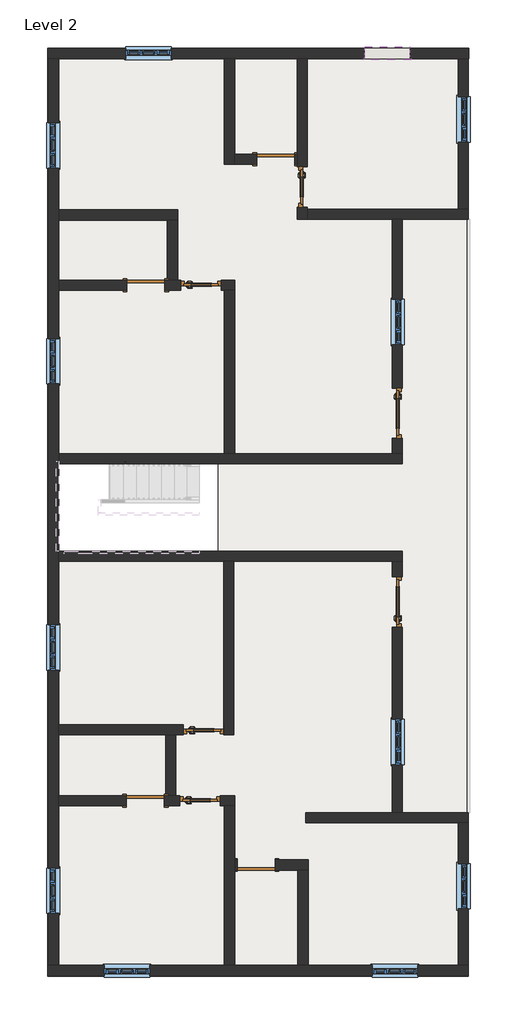
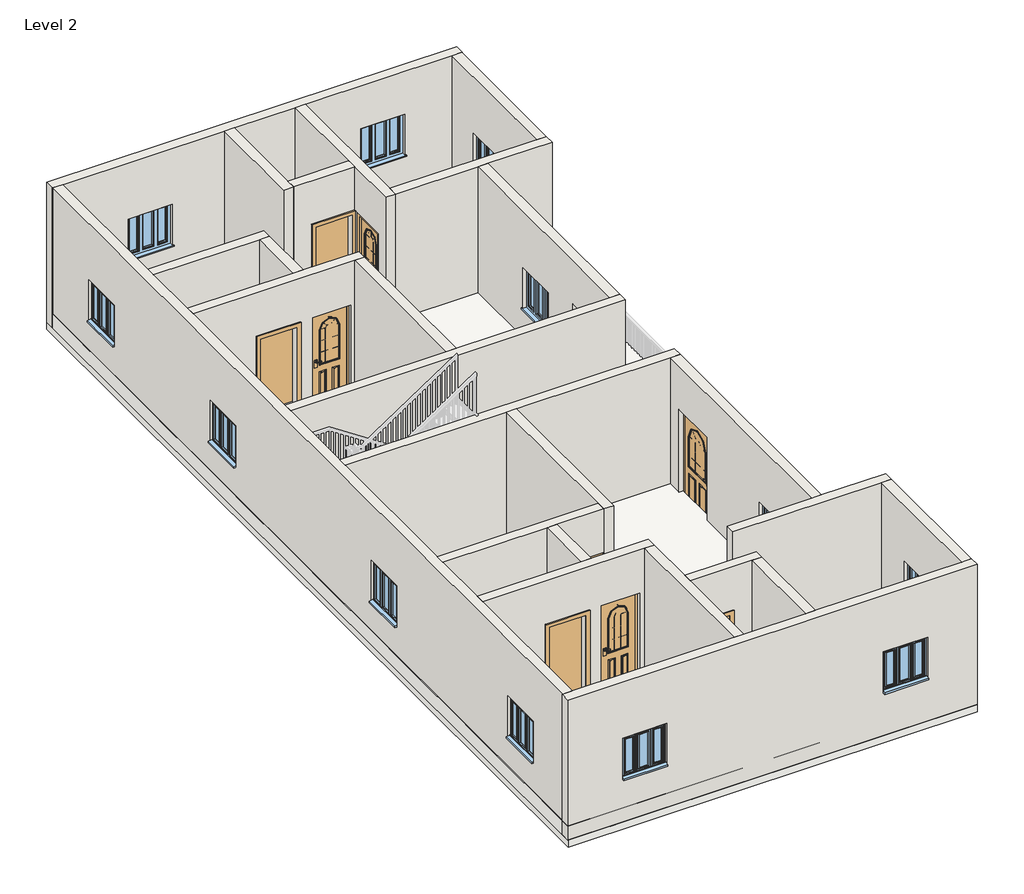
# One storey, part 1 of 3: 25 walls, 12 windows, 10 doors, 1 roof, 1 slab.
"""IFC4 building model written with IfcOpenShell, lengths in millimetres."""

from ifc_helpers import new_model, si_unit, frame, origin, place, context, project, spatial, polyline, outline, extrude, faceted_brep, transform, mapped, element, save
from components import doors_extsgl_w_glazing_bars_arched_1010x2110mm_bccdb1b2, doors_extsgl_w_glazing_bars_arched_1010x2110mm_5c897e1f, doors_extsgl_w_glazing_bars_arched_810x2110mm_57ea6d9e, doors_extsgl_w_glazing_bars_arched_810x2110mm_84a0a083, door_fadea3f2, windows_tpl_w_glazing_bars_910x910mm_9d987a72

model = new_model("IFC4")

# Units and contexts
model_context = context("Model", 3, world=origin())
ifc_project = project(units=[si_unit("LENGTHUNIT", "METRE", prefix="MILLI")], contexts=[model_context])

# Site, building, storey
site = spatial("IfcSite", under=ifc_project)
building = spatial("IfcBuilding", under=site)
storey = spatial("IfcBuildingStorey", under=building, Name="Level 2", Elevation=3048.0)

# Doors
placement = place(None, origin())
doors_extsgl_w_glazing_bars_arched_1010x2110mm_shape = doors_extsgl_w_glazing_bars_arched_1010x2110mm_bccdb1b2(model_context)
element("IfcDoor", 1, ObjectType="Doors_ExtSgl_w-Glazing_Bars_Arched : 1010x2110mm", at=placement, inside=storey, context=model_context, shape_type="MappedRepresentation", body=[
    mapped(doors_extsgl_w_glazing_bars_arched_1010x2110mm_shape, transform((1850.5605895, 2208.5797121, 3048.0), x_axis=(0.0, -1.0, 0.0), y_axis=(1.0, 0.0, 0.0), z_axis=(0.0, 0.0, 1.0))),
])
doors_extsgl_w_glazing_bars_arched_1010x2110mm_2_shape = doors_extsgl_w_glazing_bars_arched_1010x2110mm_5c897e1f(model_context)
element("IfcDoor", 2, ObjectType="Doors_ExtSgl_w-Glazing_Bars_Arched : 1010x2110mm", at=placement, inside=storey, context=model_context, shape_type="MappedRepresentation", body=[
    mapped(doors_extsgl_w_glazing_bars_arched_1010x2110mm_2_shape, transform((1850.5605895, -1576.0202879, 3048.0), x_axis=(0.0, 1.0, 0.0), y_axis=(-1.0, 0.0, 0.0), z_axis=(0.0, 0.0, 1.0))),
])
doors_extsgl_w_glazing_bars_arched_810x2110mm_shape = doors_extsgl_w_glazing_bars_arched_810x2110mm_57ea6d9e(model_context)
element("IfcDoor", 3, ObjectType="Doors_ExtSgl_w-Glazing_Bars_Arched : 810x2110mm", at=placement, inside=storey, context=model_context, shape_type="MappedRepresentation", body=[
    mapped(doors_extsgl_w_glazing_bars_arched_810x2110mm_shape, transform((-2086.4394105, 4773.9797121, 3048.0), x_axis=(1.0, 0.0, 0.0), y_axis=(0.0, 1.0, 0.0), z_axis=(0.0, 0.0, 1.0))),
])
element("IfcDoor", 4, ObjectType="Doors_ExtSgl_w-Glazing_Bars_Arched : 810x2110mm", at=placement, inside=storey, context=model_context, shape_type="MappedRepresentation", body=[
    mapped(doors_extsgl_w_glazing_bars_arched_810x2110mm_shape, transform((-2105.4894105, -5563.8202879, 3048.0), x_axis=(1.0, 0.0, 0.0), y_axis=(0.0, 1.0, 0.0), z_axis=(0.0, 0.0, 1.0))),
])
doors_extsgl_w_glazing_bars_arched_810x2110mm_2_shape = doors_extsgl_w_glazing_bars_arched_810x2110mm_84a0a083(model_context)
element("IfcDoor", 5, ObjectType="Doors_ExtSgl_w-Glazing_Bars_Arched : 810x2110mm", at=placement, inside=storey, context=model_context, shape_type="MappedRepresentation", body=[
    mapped(doors_extsgl_w_glazing_bars_arched_810x2110mm_2_shape, transform((-2035.6394105, -4141.4202879, 3048.0), x_axis=(1.0, 0.0, 0.0), y_axis=(0.0, 1.0, 0.0), z_axis=(0.0, 0.0, 1.0))),
])
element("IfcDoor", 6, ObjectType="Doors_ExtSgl_w-Glazing_Bars_Arched : 810x2110mm", at=placement, inside=storey, context=model_context, shape_type="MappedRepresentation", body=[
    mapped(doors_extsgl_w_glazing_bars_arched_810x2110mm_2_shape, transform((-54.4394105, 6748.5640518, 3048.0), x_axis=(0.0, -1.0, 0.0), y_axis=(1.0, 0.0, 0.0), z_axis=(0.0, 0.0, 1.0))),
])
door_shape = door_fadea3f2(model_context)
element("IfcDoor", 7, ObjectType="Single-Flush : 30\" x 80\"", at=placement, inside=storey, context=model_context, shape_type="MappedRepresentation", body=[
    mapped(door_shape, transform((-3204.0394105, -5563.8202879, 3048.0), x_axis=(1.0, 0.0, 0.0), y_axis=(0.0, 1.0, 0.0), z_axis=(0.0, 0.0, 1.0))),
])
element("IfcDoor", 8, ObjectType="Single-Flush : 30\" x 80\"", at=placement, inside=storey, context=model_context, shape_type="MappedRepresentation", body=[
    mapped(door_shape, transform((-981.5394105, -6850.9128362, 3048.0), x_axis=(-1.0, 0.0, 0.0), y_axis=(0.0, -1.0, 0.0), z_axis=(0.0, 0.0, 1.0))),
])
element("IfcDoor", 9, ObjectType="Single-Flush : 30\" x 80\"", at=placement, inside=storey, context=model_context, shape_type="MappedRepresentation", body=[
    mapped(door_shape, transform((-3191.3394105, 4773.9797121, 3048.0), x_axis=(1.0, 0.0, 0.0), y_axis=(0.0, 1.0, 0.0), z_axis=(0.0, 0.0, 1.0))),
])
element("IfcDoor", 10, ObjectType="Single-Flush : 30\" x 80\"", at=placement, inside=storey, context=model_context, shape_type="MappedRepresentation", body=[
    mapped(door_shape, transform((-587.8394105, 7301.2797121, 3048.0), x_axis=(1.0, 0.0, 0.0), y_axis=(0.0, 1.0, 0.0), z_axis=(0.0, 0.0, 1.0))),
])

# Roof
element("IfcRoof", 11, ObjectType="Generic - 12\"", at=placement, inside=storey, context=model_context, shape_type="SweptSolid", body=[
    extrude(outline(polyline([(3272.9605895, 9523.7797121), (3272.9605895, -9069.0202879), (-5159.8394105, -9069.0202879), (-5159.8394105, 9523.7797121), (3272.9605895, 9523.7797121)]), holes=[polyline([(-1756.1922756, 1192.5797121), (-4943.9394105, 1192.5797121), (-4943.9394105, -560.0202879), (-1756.1922756, -560.0202879), (-1756.1922756, 1192.5797121)])]), frame((0.0, 0.0, 3048.0), z_axis=(0.0, 0.0, 1.0), x_axis=(1.0, 0.0, 0.0)), (0.0, 0.0, 1.0), 304.8),
])

# Slab
element("IfcSlab", 12, ObjectType="Generic - 12\"", at=placement, inside=storey, context=model_context, shape_type="SweptSolid", body=[
    extrude(outline(polyline([(3272.9605895, 9523.7797121), (3272.9605895, -9081.7202879), (-5159.8394105, -9081.7202879), (-5159.8394105, 9523.7797121), (3272.9605895, 9523.7797121)]), holes=[polyline([(-1756.1922756, 1192.5797121), (-4943.9394105, 1192.5797121), (-4943.9394105, -560.0202879), (-1756.1922756, -560.0202879), (-1756.1922756, 1192.5797121)])]), frame((0.0, 0.0, 2895.6), z_axis=(0.0, 0.0, 1.0), x_axis=(1.0, 0.0, 0.0)), (0.0, 0.0, 1.0), 152.4),
])

# Walls
element("IfcWall", 13, ObjectType="Generic - 4.5\" p", at=placement, inside=storey, context=model_context, shape_type="Brep", body=[
    faceted_brep([(-2810.3394105, 4672.3797121, 5080.0), (-2810.3394105, 4672.3797121, 3048.0), (-2491.4394105, 4672.3797121, 3048.0), (-2491.4394105, 4672.3797121, 5158.0), (-1681.4394105, 4672.3797121, 5158.0), (-1681.4394105, 4672.3797121, 3048.0), (-1616.5394105, 4672.3797121, 3048.0), (-1413.3394105, 4672.3797121, 3048.0), (-1413.3394105, 4672.3797121, 6096.0), (-1616.5394105, 4672.3797121, 6096.0), (-4943.9394105, 4672.3797121, 6096.0), (-4943.9394105, 4672.3797121, 3048.0), (-3572.3394105, 4672.3797121, 3048.0), (-3572.3394105, 4672.3797121, 5080.0), (-2491.4394105, 4875.5797121, 3048.0), (-2556.3394105, 4875.5797121, 3048.0), (-2759.5394105, 4875.5797121, 3048.0), (-2810.3394105, 4875.5797121, 3048.0), (-2810.3394105, 4875.5797121, 5080.0), (-3572.3394105, 4875.5797121, 5080.0), (-3572.3394105, 4875.5797121, 3048.0), (-4943.9394105, 4875.5797121, 3048.0), (-4943.9394105, 4875.5797121, 6096.0), (-2759.5394105, 4875.5797121, 6096.0), (-2556.3394105, 4875.5797121, 6096.0), (-1413.3394105, 4875.5797121, 6096.0), (-1413.3394105, 4875.5797121, 3048.0), (-1681.4394105, 4875.5797121, 3048.0), (-1681.4394105, 4875.5797121, 5158.0), (-2491.4394105, 4875.5797121, 5158.0)], [[[0, 1, 2, 3, 4, 5, 6, 7, 8, 9, 10, 11, 12, 13]], [[14, 15, 16, 17, 18, 19, 20, 21, 22, 23, 24, 25, 26, 27, 28, 29]], [[7, 6, 5, 27, 26]], [[12, 11, 21, 20]], [[2, 1, 17, 16, 15, 14]], [[10, 9, 8, 25, 24, 23, 22]], [[11, 10, 22, 21]], [[8, 7, 26, 25]], [[14, 29, 3, 2]], [[28, 27, 5, 4]], [[29, 28, 4, 3]], [[18, 17, 1, 0]], [[19, 18, 0, 13]], [[20, 19, 13, 12]]]),
])
element("IfcWall", 14, ObjectType="Generic - 4.5\" p", at=placement, inside=storey, context=model_context, shape_type="SweptSolid", body=[
    extrude(outline(polyline([(-1616.5394105, 1395.7797121), (-1616.5394105, 4672.3797121), (-1413.3394105, 4672.3797121), (-1413.3394105, 1395.7797121), (-1616.5394105, 1395.7797121)])), frame((0.0, 0.0, 3048.0), z_axis=(0.0, 0.0, 1.0), x_axis=(1.0, 0.0, 0.0)), (0.0, 0.0, 1.0), 3048.0),
])
element("IfcWall", 15, ObjectType="Generic - 4.5\" p", at=placement, inside=storey, context=model_context, shape_type="Brep", body=[
    faceted_brep([(-4943.9394105, 6082.1542467, 3048.0), (-2759.5394105, 6082.1542467, 3048.0), (-2556.3394105, 6082.1542467, 3048.0), (-2556.3394105, 6082.1542467, 6096.0), (-2759.5394105, 6082.1542467, 6096.0), (-4943.9394105, 6082.1542467, 6096.0), (-4943.9394105, 6285.3542467, 3048.0), (-4943.9394105, 6285.3542467, 6096.0), (-2556.3394105, 6285.3542467, 6096.0), (-2556.3394105, 6285.3542467, 3048.0)], [[[0, 1, 2, 3, 4, 5]], [[6, 7, 8, 9]], [[2, 1, 0, 6, 9]], [[5, 4, 3, 8, 7]], [[0, 5, 7, 6]], [[3, 2, 9, 8]]]),
])
element("IfcWall", 16, ObjectType="Generic - 4.5\" p", at=placement, inside=storey, context=model_context, shape_type="SweptSolid", body=[
    extrude(outline(polyline([(-2759.5394105, 4875.5797121), (-2759.5394105, 6082.1542467), (-2556.3394105, 6082.1542467), (-2556.3394105, 4875.5797121), (-2759.5394105, 4875.5797121)])), frame((0.0, 0.0, 3048.0), z_axis=(0.0, 0.0, 1.0), x_axis=(1.0, 0.0, 0.0)), (0.0, 0.0, 1.0), 3048.0),
])
element("IfcWall", 17, ObjectType="Generic - 4.5\" p", at=placement, inside=storey, context=model_context, shape_type="Brep", body=[
    faceted_brep([(-1616.5394105, 9320.5797121, 3048.0), (-1616.5394105, 7199.6797121, 3048.0), (-1616.5394105, 7199.6797121, 6096.0), (-1616.5394105, 9320.5797121, 6096.0), (-1413.3394105, 9320.5797121, 3048.0), (-1413.3394105, 9320.5797121, 6096.0), (-1413.3394105, 7402.8797121, 6096.0), (-1413.3394105, 7199.6797121, 6096.0), (-1413.3394105, 7199.6797121, 3048.0), (-1413.3394105, 7402.8797121, 3048.0)], [[[0, 1, 2, 3]], [[4, 5, 6, 7, 8, 9]], [[1, 0, 4, 9, 8]], [[3, 2, 7, 6, 5]], [[0, 3, 5, 4]], [[2, 1, 8, 7]]]),
])
element("IfcWall", 18, ObjectType="Generic - 4.5\" p", at=placement, inside=storey, context=model_context, shape_type="SweptSolid", body=[
    extrude(outline(polyline([(5080.0, -206.8394105), (3048.0, -206.8394105), (3048.0, -156.0394105), (6096.0, -156.0394105), (6096.0, -1413.3394105), (3048.0, -1413.3394105), (3048.0, -968.8394105), (5080.0, -968.8394105), (5080.0, -206.8394105)])), frame((0.0, 7199.6797121, 0.0), z_axis=(0.0, 1.0, 0.0), x_axis=(0.0, 0.0, 1.0)), (0.0, 0.0, 1.0), 203.2),
])
element("IfcWall", 19, ObjectType="Generic - 4.5\" p", at=placement, inside=storey, context=model_context, shape_type="Brep", body=[
    faceted_brep([(-156.0394105, 6343.5640518, 5158.0), (-156.0394105, 6343.5640518, 3048.0), (-156.0394105, 6094.2483916, 3048.0), (-156.0394105, 6094.2483916, 6096.0), (-156.0394105, 7199.6797121, 6096.0), (-156.0394105, 7402.8797121, 6096.0), (-156.0394105, 9320.5797121, 6096.0), (-156.0394105, 9320.5797121, 3048.0), (-156.0394105, 7402.8797121, 3048.0), (-156.0394105, 7199.6797121, 3048.0), (-156.0394105, 7153.5640518, 3048.0), (-156.0394105, 7153.5640518, 5158.0), (47.1605895, 6094.2483916, 3048.0), (47.1605895, 6297.4483916, 3048.0), (47.1605895, 6343.5640518, 3048.0), (47.1605895, 6343.5640518, 5158.0), (47.1605895, 7153.5640518, 5158.0), (47.1605895, 7153.5640518, 3048.0), (47.1605895, 9320.5797121, 3048.0), (47.1605895, 9320.5797121, 6096.0), (47.1605895, 6297.4483916, 6096.0), (47.1605895, 6094.2483916, 6096.0)], [[[0, 1, 2, 3, 4, 5, 6, 7, 8, 9, 10, 11]], [[12, 13, 14, 15, 16, 17, 18, 19, 20, 21]], [[2, 1, 14, 13, 12]], [[10, 9, 8, 7, 18, 17]], [[6, 5, 4, 3, 21, 20, 19]], [[7, 6, 19, 18]], [[3, 2, 12, 21]], [[17, 16, 11, 10]], [[15, 14, 1, 0]], [[16, 15, 0, 11]]]),
])
element("IfcWall", 20, ObjectType="Generic - 4.5\" p", at=placement, inside=storey, context=model_context, shape_type="Brep", body=[
    faceted_brep([(47.1605895, 6094.2483916, 3048.0), (1748.9605895, 6094.2483916, 3048.0), (1952.1605895, 6094.2483916, 3048.0), (3272.9605895, 6094.2483916, 3048.0), (3272.9605895, 6094.2483916, 6096.0), (1952.1605895, 6094.2483916, 6096.0), (1748.9605895, 6094.2483916, 6096.0), (47.1605895, 6094.2483916, 6096.0), (47.1605895, 6297.4483916, 3048.0), (47.1605895, 6297.4483916, 6096.0), (3069.7605895, 6297.4483916, 6096.0), (3272.9605895, 6297.4483916, 6096.0), (3272.9605895, 6297.4483916, 3048.0), (3069.7605895, 6297.4483916, 3048.0)], [[[0, 1, 2, 3, 4, 5, 6, 7]], [[8, 9, 10, 11, 12, 13]], [[3, 2, 1, 0, 8, 13, 12]], [[7, 6, 5, 4, 11, 10, 9]], [[0, 7, 9, 8]], [[4, 3, 12, 11]]]),
])
element("IfcWall", 21, ObjectType="Generic - 4.5\" p", at=placement, inside=storey, context=model_context, shape_type="Brep", body=[
    faceted_brep([(-4943.9394105, 1192.5797121, 3048.0), (1952.1605895, 1192.5797121, 3048.0), (1952.1605895, 1192.5797121, 6096.0), (-4943.9394105, 1192.5797121, 6096.0), (-4943.9394105, 1395.7797121, 3048.0), (-4943.9394105, 1395.7797121, 6096.0), (-1616.5394105, 1395.7797121, 6096.0), (-1413.3394105, 1395.7797121, 6096.0), (1748.9605895, 1395.7797121, 6096.0), (1952.1605895, 1395.7797121, 6096.0), (1952.1605895, 1395.7797121, 3048.0), (1748.9605895, 1395.7797121, 3048.0), (-1413.3394105, 1395.7797121, 3048.0), (-1616.5394105, 1395.7797121, 3048.0)], [[[0, 1, 2, 3]], [[4, 5, 6, 7, 8, 9, 10, 11, 12, 13]], [[1, 0, 4, 13, 12, 11, 10]], [[3, 2, 9, 8, 7, 6, 5]], [[0, 3, 5, 4]], [[2, 1, 10, 9]]]),
])
element("IfcWall", 22, ObjectType="Generic - 4.5\" p", at=placement, inside=storey, context=model_context, shape_type="Brep", body=[
    faceted_brep([(-4943.9394105, -763.2202879, 3048.0), (-1629.2394105, -763.2202879, 3048.0), (-1426.0394105, -763.2202879, 3048.0), (1748.9605895, -763.2202879, 3048.0), (1952.1605895, -763.2202879, 3048.0), (1952.1605895, -763.2202879, 6096.0), (1748.9605895, -763.2202879, 6096.0), (-1426.0394105, -763.2202879, 6096.0), (-1629.2394105, -763.2202879, 6096.0), (-4943.9394105, -763.2202879, 6096.0), (-4943.9394105, -560.0202879, 3048.0), (-4943.9394105, -560.0202879, 6096.0), (1952.1605895, -560.0202879, 6096.0), (1952.1605895, -560.0202879, 3048.0)], [[[0, 1, 2, 3, 4, 5, 6, 7, 8, 9]], [[10, 11, 12, 13]], [[4, 3, 2, 1, 0, 10, 13]], [[9, 8, 7, 6, 5, 12, 11]], [[0, 9, 11, 10]], [[5, 4, 13, 12]]]),
])
element("IfcWall", 23, ObjectType="Generic - 4.5\" p", at=placement, inside=storey, context=model_context, shape_type="Brep", body=[
    faceted_brep([(-1629.2394105, -763.2202879, 3048.0), (-1629.2394105, -4039.8202879, 3048.0), (-1629.2394105, -4243.0202879, 3048.0), (-1629.2394105, -4243.0202879, 6096.0), (-1629.2394105, -4039.8202879, 6096.0), (-1629.2394105, -763.2202879, 6096.0), (-1426.0394105, -763.2202879, 3048.0), (-1426.0394105, -763.2202879, 6096.0), (-1426.0394105, -4243.0202879, 6096.0), (-1426.0394105, -4243.0202879, 3048.0)], [[[0, 1, 2, 3, 4, 5]], [[6, 7, 8, 9]], [[2, 1, 0, 6, 9]], [[5, 4, 3, 8, 7]], [[0, 5, 7, 6]], [[3, 2, 9, 8]]]),
])
element("IfcWall", 24, ObjectType="Generic - 4.5\" p", at=placement, inside=storey, context=model_context, shape_type="Brep", body=[
    faceted_brep([(-1630.6394105, -4243.0202879, 5158.0), (-1630.6394105, -4243.0202879, 3048.0), (-1629.2394105, -4243.0202879, 3048.0), (-1629.2394105, -4243.0202879, 6096.0), (-2594.4394105, -4243.0202879, 6096.0), (-2797.6394105, -4243.0202879, 6096.0), (-4943.9394105, -4243.0202879, 6096.0), (-4943.9394105, -4243.0202879, 3048.0), (-2797.6394105, -4243.0202879, 3048.0), (-2594.4394105, -4243.0202879, 3048.0), (-2440.6394105, -4243.0202879, 3048.0), (-2440.6394105, -4243.0202879, 5158.0), (-1629.2394105, -4039.8202879, 3048.0), (-1630.6394105, -4039.8202879, 3048.0), (-1630.6394105, -4039.8202879, 5158.0), (-2440.6394105, -4039.8202879, 5158.0), (-2440.6394105, -4039.8202879, 3048.0), (-4943.9394105, -4039.8202879, 3048.0), (-4943.9394105, -4039.8202879, 6096.0), (-1629.2394105, -4039.8202879, 6096.0)], [[[0, 1, 2, 3, 4, 5, 6, 7, 8, 9, 10, 11]], [[12, 13, 14, 15, 16, 17, 18, 19]], [[2, 1, 13, 12]], [[10, 9, 8, 7, 17, 16]], [[6, 5, 4, 3, 19, 18]], [[3, 2, 12, 19]], [[7, 6, 18, 17]], [[16, 15, 11, 10]], [[14, 13, 1, 0]], [[15, 14, 0, 11]]]),
])
element("IfcWall", 25, ObjectType="Generic - 4.5\" p", at=placement, inside=storey, context=model_context, shape_type="Brep", body=[
    faceted_brep([(-2823.0394105, -5665.4202879, 5080.0), (-2823.0394105, -5665.4202879, 3048.0), (-2510.4894105, -5665.4202879, 3048.0), (-2510.4894105, -5665.4202879, 5158.0), (-1700.4894105, -5665.4202879, 5158.0), (-1700.4894105, -5665.4202879, 3048.0), (-1616.5394105, -5665.4202879, 3048.0), (-1413.3394105, -5665.4202879, 3048.0), (-1413.3394105, -5665.4202879, 6096.0), (-1616.5394105, -5665.4202879, 6096.0), (-4943.9394105, -5665.4202879, 6096.0), (-4943.9394105, -5665.4202879, 3048.0), (-3585.0394105, -5665.4202879, 3048.0), (-3585.0394105, -5665.4202879, 5080.0), (-2510.4894105, -5462.2202879, 3048.0), (-2594.4394105, -5462.2202879, 3048.0), (-2797.6394105, -5462.2202879, 3048.0), (-2823.0394105, -5462.2202879, 3048.0), (-2823.0394105, -5462.2202879, 5080.0), (-3585.0394105, -5462.2202879, 5080.0), (-3585.0394105, -5462.2202879, 3048.0), (-4943.9394105, -5462.2202879, 3048.0), (-4943.9394105, -5462.2202879, 6096.0), (-2797.6394105, -5462.2202879, 6096.0), (-2594.4394105, -5462.2202879, 6096.0), (-1413.3394105, -5462.2202879, 6096.0), (-1413.3394105, -5462.2202879, 3048.0), (-1700.4894105, -5462.2202879, 3048.0), (-1700.4894105, -5462.2202879, 5158.0), (-2510.4894105, -5462.2202879, 5158.0)], [[[0, 1, 2, 3, 4, 5, 6, 7, 8, 9, 10, 11, 12, 13]], [[14, 15, 16, 17, 18, 19, 20, 21, 22, 23, 24, 25, 26, 27, 28, 29]], [[7, 6, 5, 27, 26]], [[12, 11, 21, 20]], [[2, 1, 17, 16, 15, 14]], [[10, 9, 8, 25, 24, 23, 22]], [[11, 10, 22, 21]], [[8, 7, 26, 25]], [[14, 29, 3, 2]], [[28, 27, 5, 4]], [[29, 28, 4, 3]], [[18, 17, 1, 0]], [[19, 18, 0, 13]], [[20, 19, 13, 12]]]),
])
element("IfcWall", 26, ObjectType="Generic - 4.5\" p", at=placement, inside=storey, context=model_context, shape_type="SweptSolid", body=[
    extrude(outline(polyline([(-2797.6394105, -5462.2202879), (-2797.6394105, -4243.0202879), (-2594.4394105, -4243.0202879), (-2594.4394105, -5462.2202879), (-2797.6394105, -5462.2202879)])), frame((0.0, 0.0, 3048.0), z_axis=(0.0, 0.0, 1.0), x_axis=(1.0, 0.0, 0.0)), (0.0, 0.0, 1.0), 3048.0),
])
element("IfcWall", 27, ObjectType="Generic - 4.5\" p", at=placement, inside=storey, context=model_context, shape_type="Brep", body=[
    faceted_brep([(-1616.5394105, -5665.4202879, 3048.0), (-1616.5394105, -8865.8202879, 3048.0), (-1616.5394105, -8865.8202879, 6096.0), (-1616.5394105, -5665.4202879, 6096.0), (-1413.3394105, -5665.4202879, 3048.0), (-1413.3394105, -5665.4202879, 6096.0), (-1413.3394105, -6749.3128362, 6096.0), (-1413.3394105, -6952.5128362, 6096.0), (-1413.3394105, -8865.8202879, 6096.0), (-1413.3394105, -8865.8202879, 3048.0), (-1413.3394105, -6952.5128362, 3048.0), (-1413.3394105, -6749.3128362, 3048.0)], [[[0, 1, 2, 3]], [[4, 5, 6, 7, 8, 9, 10, 11]], [[1, 0, 4, 11, 10, 9]], [[3, 2, 8, 7, 6, 5]], [[0, 3, 5, 4]], [[2, 1, 9, 8]]]),
])
element("IfcWall", 28, ObjectType="Generic - 4.5\" p", at=placement, inside=storey, context=model_context, shape_type="Brep", body=[
    faceted_brep([(-1413.3394105, -6952.5128362, 3048.0), (-1362.5394105, -6952.5128362, 3048.0), (-1362.5394105, -6952.5128362, 5080.0), (-600.5394105, -6952.5128362, 5080.0), (-600.5394105, -6952.5128362, 3048.0), (-143.3394105, -6952.5128362, 3048.0), (59.8605895, -6952.5128362, 3048.0), (59.8605895, -6952.5128362, 6096.0), (-143.3394105, -6952.5128362, 6096.0), (-1413.3394105, -6952.5128362, 6096.0), (-1362.5394105, -6749.3128362, 5080.0), (-1362.5394105, -6749.3128362, 3048.0), (-1413.3394105, -6749.3128362, 3048.0), (-1413.3394105, -6749.3128362, 6096.0), (59.8605895, -6749.3128362, 6096.0), (59.8605895, -6749.3128362, 3048.0), (-600.5394105, -6749.3128362, 3048.0), (-600.5394105, -6749.3128362, 5080.0)], [[[0, 1, 2, 3, 4, 5, 6, 7, 8, 9]], [[10, 11, 12, 13, 14, 15, 16, 17]], [[16, 15, 6, 5, 4]], [[12, 11, 1, 0]], [[9, 8, 7, 14, 13]], [[0, 9, 13, 12]], [[7, 6, 15, 14]], [[2, 1, 11, 10]], [[3, 2, 10, 17]], [[4, 3, 17, 16]]]),
])
element("IfcWall", 29, ObjectType="Generic - 4.5\" p", at=placement, inside=storey, context=model_context, shape_type="SweptSolid", body=[
    extrude(outline(polyline([(-143.3394105, -8865.8202879), (-143.3394105, -6952.5128362), (59.8605895, -6952.5128362), (59.8605895, -8865.8202879), (-143.3394105, -8865.8202879)])), frame((0.0, 0.0, 3048.0), z_axis=(0.0, 0.0, 1.0), x_axis=(1.0, 0.0, 0.0)), (0.0, 0.0, 1.0), 3048.0),
])
element("IfcWall", 30, ObjectType="Generic - 4.5\" p", at=placement, inside=storey, context=model_context, shape_type="Brep", body=[
    faceted_brep([(3272.9605895, -5805.1202879, 3048.0), (1952.1605895, -5805.1202879, 3048.0), (1748.9605895, -5805.1202879, 3048.0), (9.0605895, -5805.1202879, 3048.0), (9.0605895, -5805.1202879, 6096.0), (1748.9605895, -5805.1202879, 6096.0), (1952.1605895, -5805.1202879, 6096.0), (3272.9605895, -5805.1202879, 6096.0), (3272.9605895, -6008.3202879, 3048.0), (3272.9605895, -6008.3202879, 6096.0), (3069.7605895, -6008.3202879, 6096.0), (9.0605895, -6008.3202879, 6096.0), (9.0605895, -6008.3202879, 3048.0), (3069.7605895, -6008.3202879, 3048.0)], [[[0, 1, 2, 3, 4, 5, 6, 7]], [[8, 9, 10, 11, 12, 13]], [[3, 2, 1, 0, 8, 13, 12]], [[4, 3, 12, 11]], [[7, 6, 5, 4, 11, 10, 9]], [[0, 7, 9, 8]]]),
])
element("IfcWall", 31, ObjectType="Generic - 9\" w", at=placement, inside=storey, context=model_context, shape_type="Brep", body=[
    faceted_brep([(-5159.8394105, 9320.5797121, 3048.0), (-5147.1394105, 9320.5797121, 3048.0), (-4943.9394105, 9320.5797121, 3048.0), (-1616.5394105, 9320.5797121, 3048.0), (-1413.3394105, 9320.5797121, 3048.0), (-156.0394105, 9320.5797121, 3048.0), (47.1605895, 9320.5797121, 3048.0), (3069.7605895, 9320.5797121, 3048.0), (3272.9605895, 9320.5797121, 3048.0), (3285.6605895, 9320.5797121, 3048.0), (3285.6605895, 9320.5797121, 6096.0), (3272.9605895, 9320.5797121, 6096.0), (3069.7605895, 9320.5797121, 6096.0), (47.1605895, 9320.5797121, 6096.0), (-156.0394105, 9320.5797121, 6096.0), (-1413.3394105, 9320.5797121, 6096.0), (-1616.5394105, 9320.5797121, 6096.0), (-4943.9394105, 9320.5797121, 6096.0), (-5147.1394105, 9320.5797121, 6096.0), (-5159.8394105, 9320.5797121, 6096.0), (1192.3605895, 9320.5797121, 5158.0), (2102.3605895, 9320.5797121, 5158.0), (2102.3605895, 9320.5797121, 4248.0), (1192.3605895, 9320.5797121, 4248.0), (-3595.5394105, 9320.5797121, 4872.4), (-2685.5394105, 9320.5797121, 4872.4), (-2685.5394105, 9320.5797121, 3962.4), (-3595.5394105, 9320.5797121, 3962.4), (-5159.8394105, 9523.7797121, 3048.0), (-5159.8394105, 9523.7797121, 6096.0), (3285.6605895, 9523.7797121, 6096.0), (3285.6605895, 9523.7797121, 3048.0), (1192.3605895, 9523.7797121, 5158.0), (1192.3605895, 9523.7797121, 4248.0), (2102.3605895, 9523.7797121, 4248.0), (2102.3605895, 9523.7797121, 5158.0), (-3595.5394105, 9523.7797121, 4872.4), (-3595.5394105, 9523.7797121, 3962.4), (-2685.5394105, 9523.7797121, 3962.4), (-2685.5394105, 9523.7797121, 4872.4)], [[[0, 1, 2, 3, 4, 5, 6, 7, 8, 9, 10, 11, 12, 13, 14, 15, 16, 17, 18, 19], [20, 21, 22, 23], [24, 25, 26, 27]], [[28, 29, 30, 31], [32, 33, 34, 35], [36, 37, 38, 39]], [[9, 8, 7, 6, 5, 4, 3, 2, 1, 0, 28, 31]], [[10, 9, 31, 30]], [[19, 18, 17, 16, 15, 14, 13, 12, 11, 10, 30, 29]], [[0, 19, 29, 28]], [[33, 32, 20, 23]], [[34, 33, 23, 22]], [[35, 34, 22, 21]], [[32, 35, 21, 20]], [[37, 36, 24, 27]], [[38, 37, 27, 26]], [[39, 38, 26, 25]], [[36, 39, 25, 24]]]),
])
element("IfcWall", 32, ObjectType="Generic - 9\" w", at=placement, inside=storey, context=model_context, shape_type="Brep", body=[
    faceted_brep([(3272.9605895, -8865.8202879, 3048.0), (3069.7605895, -8865.8202879, 3048.0), (59.8605895, -8865.8202879, 3048.0), (-143.3394105, -8865.8202879, 3048.0), (-1413.3394105, -8865.8202879, 3048.0), (-1616.5394105, -8865.8202879, 3048.0), (-4943.9394105, -8865.8202879, 3048.0), (-5147.1394105, -8865.8202879, 3048.0), (-5159.8394105, -8865.8202879, 3048.0), (-5159.8394105, -8865.8202879, 6096.0), (-5147.1394105, -8865.8202879, 6096.0), (-4943.9394105, -8865.8202879, 6096.0), (-1616.5394105, -8865.8202879, 6096.0), (-1413.3394105, -8865.8202879, 6096.0), (-143.3394105, -8865.8202879, 6096.0), (59.8605895, -8865.8202879, 6096.0), (3069.7605895, -8865.8202879, 6096.0), (3272.9605895, -8865.8202879, 6096.0), (-3117.3394105, -8865.8202879, 4872.4), (-4027.3394105, -8865.8202879, 4872.4), (-4027.3394105, -8865.8202879, 3962.4), (-3117.3394105, -8865.8202879, 3962.4), (2254.7605895, -8865.8202879, 4872.4), (1344.7605895, -8865.8202879, 4872.4), (1344.7605895, -8865.8202879, 3962.4), (2254.7605895, -8865.8202879, 3962.4), (3272.9605895, -9069.0202879, 3048.0), (3272.9605895, -9069.0202879, 6096.0), (-5159.8394105, -9069.0202879, 6096.0), (-5159.8394105, -9069.0202879, 3048.0), (-3117.3394105, -9069.0202879, 4872.4), (-3117.3394105, -9069.0202879, 3962.4), (-4027.3394105, -9069.0202879, 3962.4), (-4027.3394105, -9069.0202879, 4872.4), (2254.7605895, -9069.0202879, 4872.4), (2254.7605895, -9069.0202879, 3962.4), (1344.7605895, -9069.0202879, 3962.4), (1344.7605895, -9069.0202879, 4872.4)], [[[0, 1, 2, 3, 4, 5, 6, 7, 8, 9, 10, 11, 12, 13, 14, 15, 16, 17], [18, 19, 20, 21], [22, 23, 24, 25]], [[26, 27, 28, 29], [30, 31, 32, 33], [34, 35, 36, 37]], [[8, 7, 6, 5, 4, 3, 2, 1, 0, 26, 29]], [[9, 8, 29, 28]], [[17, 16, 15, 14, 13, 12, 11, 10, 9, 28, 27]], [[0, 17, 27, 26]], [[31, 30, 18, 21]], [[32, 31, 21, 20]], [[33, 32, 20, 19]], [[30, 33, 19, 18]], [[35, 34, 22, 25]], [[36, 35, 25, 24]], [[37, 36, 24, 23]], [[34, 37, 23, 22]]]),
])
element("IfcWall", 33, ObjectType="Generic - 9\" w", at=placement, inside=storey, context=model_context, shape_type="Brep", body=[
    faceted_brep([(-4943.9394105, -8865.8202879, 3048.0), (-4943.9394105, -5665.4202879, 3048.0), (-4943.9394105, -5462.2202879, 3048.0), (-4943.9394105, -4243.0202879, 3048.0), (-4943.9394105, -4039.8202879, 3048.0), (-4943.9394105, -763.2202879, 3048.0), (-4943.9394105, -560.0202879, 3048.0), (-4943.9394105, 1192.5797121, 3048.0), (-4943.9394105, 1395.7797121, 3048.0), (-4943.9394105, 4672.3797121, 3048.0), (-4943.9394105, 4875.5797121, 3048.0), (-4943.9394105, 6082.1542467, 3048.0), (-4943.9394105, 6285.3542467, 3048.0), (-4943.9394105, 9320.5797121, 3048.0), (-4943.9394105, 9320.5797121, 6096.0), (-4943.9394105, 6285.3542467, 6096.0), (-4943.9394105, 6082.1542467, 6096.0), (-4943.9394105, 4875.5797121, 6096.0), (-4943.9394105, 4672.3797121, 6096.0), (-4943.9394105, 1395.7797121, 6096.0), (-4943.9394105, 1192.5797121, 6096.0), (-4943.9394105, -560.0202879, 6096.0), (-4943.9394105, -763.2202879, 6096.0), (-4943.9394105, -4039.8202879, 6096.0), (-4943.9394105, -4243.0202879, 6096.0), (-4943.9394105, -5462.2202879, 6096.0), (-4943.9394105, -5665.4202879, 6096.0), (-4943.9394105, -8865.8202879, 6096.0), (-4943.9394105, -7822.2202879, 4872.4), (-4943.9394105, -6912.2202879, 4872.4), (-4943.9394105, -6912.2202879, 3962.4), (-4943.9394105, -7822.2202879, 3962.4), (-4943.9394105, -2945.4202879, 4872.4), (-4943.9394105, -2035.4202879, 4872.4), (-4943.9394105, -2035.4202879, 3962.4), (-4943.9394105, -2945.4202879, 3962.4), (-4943.9394105, 2794.9797121, 4872.4), (-4943.9394105, 3704.9797121, 4872.4), (-4943.9394105, 3704.9797121, 3962.4), (-4943.9394105, 2794.9797121, 3962.4), (-4943.9394105, 7125.7542467, 4872.4), (-4943.9394105, 8035.7542467, 4872.4), (-4943.9394105, 8035.7542467, 3962.4), (-4943.9394105, 7125.7542467, 3962.4), (-5147.1394105, -8865.8202879, 3048.0), (-5147.1394105, -8865.8202879, 6096.0), (-5147.1394105, 9320.5797121, 6096.0), (-5147.1394105, 9320.5797121, 3048.0), (-5147.1394105, -7822.2202879, 4872.4), (-5147.1394105, -7822.2202879, 3962.4), (-5147.1394105, -6912.2202879, 3962.4), (-5147.1394105, -6912.2202879, 4872.4), (-5147.1394105, -2945.4202879, 4872.4), (-5147.1394105, -2945.4202879, 3962.4), (-5147.1394105, -2035.4202879, 3962.4), (-5147.1394105, -2035.4202879, 4872.4), (-5147.1394105, 2794.9797121, 4872.4), (-5147.1394105, 2794.9797121, 3962.4), (-5147.1394105, 3704.9797121, 3962.4), (-5147.1394105, 3704.9797121, 4872.4), (-5147.1394105, 7125.7542467, 4872.4), (-5147.1394105, 7125.7542467, 3962.4), (-5147.1394105, 8035.7542467, 3962.4), (-5147.1394105, 8035.7542467, 4872.4)], [[[0, 1, 2, 3, 4, 5, 6, 7, 8, 9, 10, 11, 12, 13, 14, 15, 16, 17, 18, 19, 20, 21, 22, 23, 24, 25, 26, 27], [28, 29, 30, 31], [32, 33, 34, 35], [36, 37, 38, 39], [40, 41, 42, 43]], [[44, 45, 46, 47], [48, 49, 50, 51], [52, 53, 54, 55], [56, 57, 58, 59], [60, 61, 62, 63]], [[13, 12, 11, 10, 9, 8, 7, 6, 5, 4, 3, 2, 1, 0, 44, 47]], [[27, 26, 25, 24, 23, 22, 21, 20, 19, 18, 17, 16, 15, 14, 46, 45]], [[14, 13, 47, 46]], [[0, 27, 45, 44]], [[49, 48, 28, 31]], [[50, 49, 31, 30]], [[51, 50, 30, 29]], [[48, 51, 29, 28]], [[53, 52, 32, 35]], [[54, 53, 35, 34]], [[55, 54, 34, 33]], [[52, 55, 33, 32]], [[57, 56, 36, 39]], [[58, 57, 39, 38]], [[59, 58, 38, 37]], [[56, 59, 37, 36]], [[61, 60, 40, 43]], [[62, 61, 43, 42]], [[63, 62, 42, 41]], [[60, 63, 41, 40]]]),
])
element("IfcWall", 34, ObjectType="Generic - 9\" w", at=placement, inside=storey, context=model_context, shape_type="SweptSolid", body=[
    extrude(outline(polyline([(-8865.8202879, 3048.0), (-8865.8202879, 6096.0), (-6008.3202879, 6096.0), (-6008.3202879, 3048.0), (-8865.8202879, 3048.0)]), holes=[polyline([(-6823.3202879, 4872.4), (-7733.3202879, 4872.4), (-7733.3202879, 3962.4), (-6823.3202879, 3962.4), (-6823.3202879, 4872.4)])]), frame((3069.7605895, 0.0, 0.0), z_axis=(1.0, 0.0, 0.0), x_axis=(0.0, 1.0, 0.0)), (0.0, 0.0, 1.0), 203.2),
])
element("IfcWall", 35, ObjectType="Generic - 9\" w", at=placement, inside=storey, context=model_context, shape_type="SweptSolid", body=[
    extrude(outline(polyline([(9320.5797121, 3048.0), (6297.4483916, 3048.0), (6297.4483916, 6096.0), (9320.5797121, 6096.0), (9320.5797121, 3048.0)]), holes=[polyline([(8556.3797121, 4872.4), (7646.3797121, 4872.4), (7646.3797121, 3962.4), (8556.3797121, 3962.4), (8556.3797121, 4872.4)])]), frame((3069.7605895, 0.0, 0.0), z_axis=(1.0, 0.0, 0.0), x_axis=(0.0, 1.0, 0.0)), (0.0, 0.0, 1.0), 203.2),
])
element("IfcWall", 36, ObjectType="Generic - 9\" w", at=placement, inside=storey, context=model_context, shape_type="SweptSolid", body=[
    extrude(outline(polyline([(-763.2202879, 3048.0), (-1071.0202879, 3048.0), (-1071.0202879, 5158.0), (-2081.0202879, 5158.0), (-2081.0202879, 3048.0), (-5805.1202879, 3048.0), (-5805.1202879, 6096.0), (-763.2202879, 6096.0), (-763.2202879, 3048.0)]), holes=[polyline([(-3927.7202879, 4872.4), (-4837.7202879, 4872.4), (-4837.7202879, 3962.4), (-3927.7202879, 3962.4), (-3927.7202879, 4872.4)])]), frame((1748.9605895, 0.0, 0.0), z_axis=(1.0, 0.0, 0.0), x_axis=(0.0, 1.0, 0.0)), (0.0, 0.0, 1.0), 203.2),
])
element("IfcWall", 37, ObjectType="Generic - 9\" w", at=placement, inside=storey, context=model_context, shape_type="SweptSolid", body=[
    extrude(outline(polyline([(1703.5797121, 5158.0), (1703.5797121, 3048.0), (1395.7797121, 3048.0), (1395.7797121, 6096.0), (6094.2483916, 6096.0), (6094.2483916, 3048.0), (2713.5797121, 3048.0), (2713.5797121, 5158.0), (1703.5797121, 5158.0)]), holes=[polyline([(4492.3797121, 4872.4), (3582.3797121, 4872.4), (3582.3797121, 3962.4), (4492.3797121, 3962.4), (4492.3797121, 4872.4)])]), frame((1748.9605895, 0.0, 0.0), z_axis=(1.0, 0.0, 0.0), x_axis=(0.0, 1.0, 0.0)), (0.0, 0.0, 1.0), 203.2),
])

# Windows
windows_tpl_w_glazing_bars_910x910mm_shape = windows_tpl_w_glazing_bars_910x910mm_9d987a72(model_context)
element("IfcWindow", 38, ObjectType="Windows_Tpl_w-Glazing_Bars : 910x910mm", at=placement, inside=storey, context=model_context, shape_type="MappedRepresentation", body=[
    mapped(windows_tpl_w_glazing_bars_910x910mm_shape, transform((-3809.0060772, -8958.9637201, 2762.4), x_axis=(-1.0, 0.0, 0.0), y_axis=(0.0, -1.0, 0.0), z_axis=(0.0, 0.0, 1.0))),
])
element("IfcWindow", 39, ObjectType="Windows_Tpl_w-Glazing_Bars : 910x910mm", at=placement, inside=storey, context=model_context, shape_type="MappedRepresentation", body=[
    mapped(windows_tpl_w_glazing_bars_910x910mm_shape, transform((-5037.0828427, -7130.5536213, 2762.4), x_axis=(0.0, 1.0, 0.0), y_axis=(-1.0, 0.0, 0.0), z_axis=(0.0, 0.0, 1.0))),
])
element("IfcWindow", 40, ObjectType="Windows_Tpl_w-Glazing_Bars : 910x910mm", at=placement, inside=storey, context=model_context, shape_type="MappedRepresentation", body=[
    mapped(windows_tpl_w_glazing_bars_910x910mm_shape, transform((-5037.0828427, -2253.7536213, 2762.4), x_axis=(0.0, 1.0, 0.0), y_axis=(-1.0, 0.0, 0.0), z_axis=(0.0, 0.0, 1.0))),
])
element("IfcWindow", 41, ObjectType="Windows_Tpl_w-Glazing_Bars : 910x910mm", at=placement, inside=storey, context=model_context, shape_type="MappedRepresentation", body=[
    mapped(windows_tpl_w_glazing_bars_910x910mm_shape, transform((-5037.0828427, 3486.6463787, 2762.4), x_axis=(0.0, 1.0, 0.0), y_axis=(-1.0, 0.0, 0.0), z_axis=(0.0, 0.0, 1.0))),
])
element("IfcWindow", 42, ObjectType="Windows_Tpl_w-Glazing_Bars : 910x910mm", at=placement, inside=storey, context=model_context, shape_type="MappedRepresentation", body=[
    mapped(windows_tpl_w_glazing_bars_910x910mm_shape, transform((3162.9040216, 7864.7130454, 2762.4), x_axis=(0.0, -1.0, 0.0), y_axis=(1.0, 0.0, 0.0), z_axis=(0.0, 0.0, 1.0))),
])
element("IfcWindow", 43, ObjectType="Windows_Tpl_w-Glazing_Bars : 910x910mm", at=placement, inside=storey, context=model_context, shape_type="MappedRepresentation", body=[
    mapped(windows_tpl_w_glazing_bars_910x910mm_shape, transform((1884.0272561, 9413.7231443, 3048.0), x_axis=(1.0, 0.0, 0.0), y_axis=(0.0, 1.0, 0.0), z_axis=(0.0, 0.0, 1.0))),
])
element("IfcWindow", 44, ObjectType="Windows_Tpl_w-Glazing_Bars : 910x910mm", at=placement, inside=storey, context=model_context, shape_type="MappedRepresentation", body=[
    mapped(windows_tpl_w_glazing_bars_910x910mm_shape, transform((1563.0939228, -8958.9637201, 2762.4), x_axis=(-1.0, 0.0, 0.0), y_axis=(0.0, -1.0, 0.0), z_axis=(0.0, 0.0, 1.0))),
])
element("IfcWindow", 45, ObjectType="Windows_Tpl_w-Glazing_Bars : 910x910mm", at=placement, inside=storey, context=model_context, shape_type="MappedRepresentation", body=[
    mapped(windows_tpl_w_glazing_bars_910x910mm_shape, transform((3162.9040216, -7514.9869546, 2762.4), x_axis=(0.0, -1.0, 0.0), y_axis=(1.0, 0.0, 0.0), z_axis=(0.0, 0.0, 1.0))),
])
element("IfcWindow", 46, ObjectType="Windows_Tpl_w-Glazing_Bars : 910x910mm", at=placement, inside=storey, context=model_context, shape_type="MappedRepresentation", body=[
    mapped(windows_tpl_w_glazing_bars_910x910mm_shape, transform((-5037.0828427, 7817.4209133, 2762.4), x_axis=(0.0, 1.0, 0.0), y_axis=(-1.0, 0.0, 0.0), z_axis=(0.0, 0.0, 1.0))),
])
element("IfcWindow", 47, ObjectType="Windows_Tpl_w-Glazing_Bars : 910x910mm", at=placement, inside=storey, context=model_context, shape_type="MappedRepresentation", body=[
    mapped(windows_tpl_w_glazing_bars_910x910mm_shape, transform((-2903.8727439, 9413.7231443, 2762.4), x_axis=(1.0, 0.0, 0.0), y_axis=(0.0, 1.0, 0.0), z_axis=(0.0, 0.0, 1.0))),
])
element("IfcWindow", 48, ObjectType="Windows_Tpl_w-Glazing_Bars : 910x910mm", at=placement, inside=storey, context=model_context, shape_type="MappedRepresentation", body=[
    mapped(windows_tpl_w_glazing_bars_910x910mm_shape, transform((1842.1040216, -4619.3869546, 2762.4), x_axis=(0.0, -1.0, 0.0), y_axis=(1.0, 0.0, 0.0), z_axis=(0.0, 0.0, 1.0))),
])
element("IfcWindow", 49, ObjectType="Windows_Tpl_w-Glazing_Bars : 910x910mm", at=placement, inside=storey, context=model_context, shape_type="MappedRepresentation", body=[
    mapped(windows_tpl_w_glazing_bars_910x910mm_shape, transform((1842.1040216, 3800.7130454, 2762.4), x_axis=(0.0, -1.0, 0.0), y_axis=(1.0, 0.0, 0.0), z_axis=(0.0, 0.0, 1.0))),
])

save(model, "model.ifc")

# Revit data of these elements
# Type "Doors_ExtSgl_w-Glazing_Bars_Arched : 1010x2110mm"
#   Type Mark = "10"
#   Type Comments = "External Single"
#   Operation = "SingleSwingRight"
#   Construction Type Id = "SGL"
#   Keynote = "L20"
#   Analytic Construction = "Large single-glazed windows"
#   Wrap Layers (Int) from Ext = 177.5 mm
#   Wrap Layers (Ext) from Ext = 102.5 mm
#   Visual Light Transmittance = 0.9
#   Thickness = 44 mm
#   Solar Heat Gain Coefficient = 0.86
#   Rough Width = 1010 mm
#   Rough Height = 2110 mm
#   O/A Frame Width = 64 mm
#   Heat Transfer Coefficient (U) = 0.979472 BTU/(h·ft²·°F)
#   Handle Z Distance = 1050 mm
#   Glazing Thickness = 24 mm
#   FrameWidth = 42 mm
#   FrameOffset - External = 25 mm
#   FrameDepth = 89 mm
#   Door Panel Width = 907 mm
#   Door Panel Thickness = 44 mm
#   Door Panel Height = 2000 mm
#   DONT CHANGE - Half Glazed Width = 303.5 mm
#   DONT CHANGE - Glazed Width = 607 mm
#   Cill Thickness = 54.5 mm
#   Cill Projection = 30 mm
#   Handle X Distance = 75 mm
#   Height = 2110 mm
#   Structural Tolerance = 6.5 mm
#   Tolerance = 3 mm
#   Undercut = 4 mm
#   Width = 1010 mm
#   Cill Extension = 25 mm
#   Cavity Closer Width = 50 mm
#   Cavity Closer Offset from Ext = 102.5 mm
#   Cavity Closer Depth = 85 mm
#   Vis - Ironmongery = yes
#   Vis - Glazing Bars = yes
#   Vis - Cavity Closers = yes
#   Define Thermal Properties by = 1
#   Function = 1
#   Material Glass = Door - Glazing
#   Material Glazing Bar = Door - Panel
#   Material Door = Door - Panel
#   Material Frame = Door - Frame/Mullion
#   Material Ironmongery = Door - Handle
#   Wall Closure = (empty or 0)
# Type "Doors_ExtSgl_w-Glazing_Bars_Arched : 810x2110mm"
#   Type Mark = "9"
#   Type Comments = "External Single"
#   Operation = "SingleSwingRight"
#   Construction Type Id = "SGL"
#   Keynote = "L20"
#   Analytic Construction = "Large single-glazed windows"
#   Wrap Layers (Int) from Ext = 177.5 mm
#   Wrap Layers (Ext) from Ext = 102.5 mm
#   Visual Light Transmittance = 0.9
#   Thickness = 44 mm
#   Solar Heat Gain Coefficient = 0.86
#   Rough Width = 810 mm
#   Rough Height = 2110 mm
#   O/A Frame Width = 64 mm
#   Heat Transfer Coefficient (U) = 0.979472 BTU/(h·ft²·°F)
#   Handle Z Distance = 1050 mm
#   Glazing Thickness = 24 mm
#   FrameWidth = 42 mm
#   FrameOffset - External = 25 mm
#   FrameDepth = 89 mm
#   Door Panel Width = 707 mm
#   Door Panel Thickness = 44 mm
#   Door Panel Height = 2000 mm
#   DONT CHANGE - Half Glazed Width = 203.5 mm
#   DONT CHANGE - Glazed Width = 407 mm
#   Cill Thickness = 54.5 mm
#   Cill Projection = 30 mm
#   Handle X Distance = 75 mm
#   Height = 2110 mm
#   Structural Tolerance = 6.5 mm
#   Tolerance = 3 mm
#   Undercut = 4 mm
#   Width = 810 mm
#   Cill Extension = 25 mm
#   Cavity Closer Width = 50 mm
#   Cavity Closer Offset from Ext = 102.5 mm
#   Cavity Closer Depth = 85 mm
#   Vis - Ironmongery = yes
#   Vis - Glazing Bars = yes
#   Vis - Cavity Closers = yes
#   Define Thermal Properties by = 1
#   Function = 1
#   Material Glass = Door - Glazing
#   Material Glazing Bar = Door - Panel
#   Material Door = Door - Panel
#   Material Frame = Door - Frame/Mullion
#   Material Ironmongery = Door - Handle
#   Wall Closure = (empty or 0)
# Type "Single-Flush : 30\" x 80\""
#   Type Mark = "5"
#   Construction Type Id = "MDOOR"
#   Assembly Code = "C1020"
#   Analytic Construction = "Metal"
#   Thickness = 50.8 mm
#   Heat Transfer Coefficient (U) = 0.651978 BTU/(h·ft²·°F)
#   Height = 2032 mm
#   Trim Projection Ext = 25.4 mm
#   Trim Projection Int = 25.4 mm
#   Trim Width = 76.2 mm
#   Width = 762 mm
#   Define Thermal Properties by = 1
#   Define Thermal Properties by = 1
#   Door Material = Door - Panel
#   Frame Material = Door - Frame
#   Visual Light Transmittance = 0
#   Solar Heat Gain Coefficient = 0
#   Function = (empty or 0)
#   Wall Closure = (empty or 0)
# Type "Generic - 12\""
#   Assembly Code = "B1020"
#   Layers, outside or top first: 304.8 mm no material (function 1)
# Type "Generic - 12\""
#   Assembly Code = "B1010"
#   Function = 0
#   Layers, outside or top first: 152.4 mm no material (function 1)
# Type "Generic - 4.5\" p"
#   Assembly Code = "B2010"
#   Layers, outside or top first: 203.2 mm no material (function 1)
# Type "Generic - 9\" w"
#   Assembly Code = "B2010"
#   Layers, outside or top first: 203.2 mm no material (function 1)
# Type "Windows_Tpl_w-Glazing_Bars : 910x910mm"
#   Type Mark = "18"
#   Operation = "TriplePanelVertical"
#   Construction Type Id = "GSP4R"
#   Manufacturer = "Revit"
#   Keynote = "L10"
#   Analytic Construction = "1/8 in Pilkington single glazing"
#   Length 1 = 24 mm
#   Wrap Layers (Ext) from Ext = 102.5 mm
#   Wrap Layers (Int) from Ext = 177.5 mm
#   Window Board Projection = 25 mm
#   Window Board Extension = 25 mm
#   Visual Light Transmittance = 0.9
#   Solar Heat Gain Coefficient = 0.78
#   Rough Width = 910 mm
#   Rough Height = 910 mm
#   Height = 910 mm
#   Width = 910 mm
#   Heat Transfer Coefficient (U) = 0.6496 BTU/(h·ft²·°F)
#   Glazing Thickness = 24 mm
#   Glazing Bar Thickness = 20 mm
#   FrameOffset - External = 50 mm
#   Frame Depth = 65 mm
#   Default Head Height = 2110 mm
#   Cill Depth = 87.5 mm
#   Cavity Closer Width = 50 mm
#   Cavity Closer Offset from Ext = 102.5 mm
#   Cavity Closer Depth = 85 mm
#   Vis - Glazing Bars = yes
#   Vis - Cavity Closers = yes
#   Define Thermal Properties by = 1
#   Material Trim = Window Frame
#   Material Glazing Bars = Window Frame
#   Material Glass = Glass
#   Material Frame = Window Frame
#   Wall Closure = (empty or 0)
# Elements 1, 2 (IfcDoor, "Doors_ExtSgl_w-Glazing_Bars_Arched : 1010x2110mm")
#   Phase Created = New Construction
#   Materials on its faces: "Door - Panel", "Door - Handle", "Door - Frame/Mullion", "Door - Glazing"
# Elements 3, 4, 5, 6 (IfcDoor, "Doors_ExtSgl_w-Glazing_Bars_Arched : 810x2110mm")
#   Phase Created = New Construction
#   Materials on its faces: "Door - Panel", "Door - Handle", "Door - Frame/Mullion", "Door - Glazing"
# Elements 7, 8, 9, 10 (IfcDoor, "Single-Flush : 30\" x 80\"")
#   Phase Created = New Construction
#   Materials on its faces: "Door - Frame", "Door - Panel"
# Element 11 (IfcRoof, "Generic - 12\"")
#   built-in parameter 1001705 = 11 (stored number, unit not read)
#   built-in parameter 1001710 = 33615
#   Phase Created = New Construction
#   Materials on its faces: "Default Roof", "Door - Frame", "Wood Planks"
# Element 12 (IfcSlab, "Generic - 12\"")
#   Height Offset From Level = 0 mm
#   Phase Created = New Construction
#   Materials on its faces: "Default Floor", "Wood Planks"
# Elements 13, 14, 15, 16, 17, 18, 19, 23, 24, 25, 26, 27, 28, 29 (IfcWall, "Generic - 4.5\" p")
#   Top Offset = 0 mm
#   Base Offset = 0 mm
#   wall height = 3048 mm
#   Phase Created = New Construction
#   Base Constraint = Level 2
#   Top Constraint = Level 3
#   Materials on its faces: "Default Wall"
# Elements 20, 30 (IfcWall, "Generic - 4.5\" p")
#   Top Offset = 0 mm
#   Base Offset = 0 mm
#   wall height = 3048 mm
#   Phase Created = New Construction
#   Base Constraint = Level 2
#   Top Constraint = Level 3
#   Materials on its faces: "Default Wall", "Default Mass Interior Wall"
# Elements 21, 22 (IfcWall, "Generic - 4.5\" p")
#   Top Offset = 0 mm
#   Base Offset = 0 mm
#   wall height = 3048 mm
#   Phase Created = New Construction
#   Base Constraint = Level 2
#   Top Constraint = Level 3
#   Materials on its faces: "Default Wall", "Window Frame", "Wood Planks"
# Elements 31, 32 (IfcWall, "Generic - 9\" w")
#   Top Offset = 0 mm
#   Base Offset = 0 mm
#   wall height = 3048 mm
#   Phase Created = New Construction
#   Base Constraint = Level 2
#   Top Constraint = Level 3
#   Materials on its faces: "Default Wall", "Wood Planks", "Default Mass Interior Wall"
# Elements 33, 36, 37 (IfcWall, "Generic - 9\" w")
#   Top Offset = 0 mm
#   Base Offset = 0 mm
#   wall height = 3048 mm
#   Phase Created = New Construction
#   Base Constraint = Level 2
#   Top Constraint = Level 3
#   Materials on its faces: "Default Wall", "Wood Planks"
# Elements 34, 35 (IfcWall, "Generic - 9\" w")
#   Top Offset = 0 mm
#   Base Offset = 0 mm
#   wall height = 3048 mm
#   Phase Created = New Construction
#   Base Constraint = Level 2
#   Top Constraint = Level 3
#   Materials on its faces: "Default Wall", "Default Mass Interior Wall"
# Element 38 (IfcWindow, "Windows_Tpl_w-Glazing_Bars : 910x910mm")
#   Mark = "16"
#   Phase Created = New Construction
#   Materials on its faces: "Window Frame", "Glass"
# Element 39 (IfcWindow, "Windows_Tpl_w-Glazing_Bars : 910x910mm")
#   Mark = "17"
#   Phase Created = New Construction
#   Materials on its faces: "Window Frame", "Glass"
# Element 40 (IfcWindow, "Windows_Tpl_w-Glazing_Bars : 910x910mm")
#   Mark = "18"
#   Phase Created = New Construction
#   Materials on its faces: "Window Frame", "Glass"
# Element 41 (IfcWindow, "Windows_Tpl_w-Glazing_Bars : 910x910mm")
#   Mark = "19"
#   Phase Created = New Construction
#   Materials on its faces: "Window Frame", "Glass"
# Element 42 (IfcWindow, "Windows_Tpl_w-Glazing_Bars : 910x910mm")
#   Mark = "20"
#   Phase Created = New Construction
#   Materials on its faces: "Window Frame", "Glass"
# Element 43 (IfcWindow, "Windows_Tpl_w-Glazing_Bars : 910x910mm")
#   Mark = "21"
#   Phase Created = New Construction
#   Materials on its faces: "Window Frame", "Glass"
# Element 44 (IfcWindow, "Windows_Tpl_w-Glazing_Bars : 910x910mm")
#   Mark = "22"
#   Phase Created = New Construction
#   Materials on its faces: "Window Frame", "Glass"
# Element 45 (IfcWindow, "Windows_Tpl_w-Glazing_Bars : 910x910mm")
#   Mark = "23"
#   Phase Created = New Construction
#   Materials on its faces: "Window Frame", "Glass"
# Element 46 (IfcWindow, "Windows_Tpl_w-Glazing_Bars : 910x910mm")
#   Mark = "24"
#   Phase Created = New Construction
#   Materials on its faces: "Window Frame", "Glass"
# Element 47 (IfcWindow, "Windows_Tpl_w-Glazing_Bars : 910x910mm")
#   Mark = "25"
#   Phase Created = New Construction
#   Materials on its faces: "Window Frame", "Glass"
# Element 48 (IfcWindow, "Windows_Tpl_w-Glazing_Bars : 910x910mm")
#   Mark = "26"
#   Phase Created = New Construction
#   Materials on its faces: "Window Frame", "Glass"
# Element 49 (IfcWindow, "Windows_Tpl_w-Glazing_Bars : 910x910mm")
#   Mark = "27"
#   Phase Created = New Construction
#   Materials on its faces: "Window Frame", "Glass"
# Materials
#   "Door - Glazing": colour RGB 0 0 255, transparency 0.75
#   "Door - Panel": class "Wood", colour RGB 210 159 95, transparency 0, Cost = 0
#   "Door - Frame/Mullion": class "Wood", colour RGB 212 179 113, transparency 0
#   "Door - Handle": colour RGB 246 240 166, transparency 0
#   "Door - Frame": colour RGB 118 70 51, transparency 0, Cost = 0
#   "Window Frame": colour RGB 249 249 249, transparency 0
#   "Glass": class "Glass", colour RGB 0 128 192, transparency 0.75, Description = "Soda Lime Glass", Cost = 0
#   "Default Roof": colour RGB 88 101 114, transparency 0, Cost = 0
#   "Wood Planks": class "Wood", colour RGB 193 160 115, transparency 0, Description = "Physical material.", Cost = 0
#   "Default Floor": colour RGB 128 128 128, transparency 0, Cost = 0
#   "Default Wall": colour RGB 128 128 128, transparency 0, Cost = 0
#   "Default Mass Interior Wall": class "Generic", colour RGB 195 229 126, transparency 0, Cost = 0
